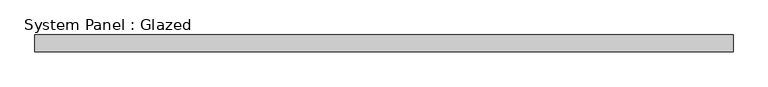
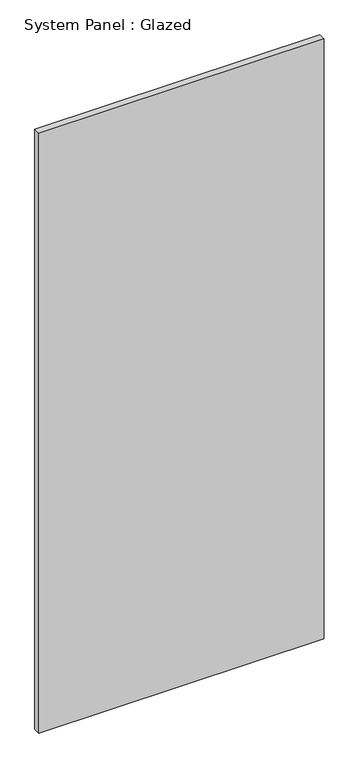
"""IFC4 building model written with IfcOpenShell, lengths in millimetres: plate geometry, System Panel : Glazed."""

from ifc_helpers import new_model, si_unit, origin, origin_with_axes, place, context, project, spatial, polyline, outline, extrude, source, transform, mapped, element, save


def system_panel_glazed_0266aec6(model_context):
    return source(origin(), model_context, "Body", "SweptSolid", [
        extrude(outline(polyline([(527.05, 19.05), (-527.05, 19.05), (-527.05, 44.45), (527.05, 44.45), (527.05, 19.05)])), origin_with_axes(), (0.0, 0.0, 1.0), 2343.15),
    ])


if __name__ == "__main__":
    model = new_model("IFC4")
    model_context = context("Model", 3, world=origin())
    ifc_project = project(units=[si_unit("LENGTHUNIT", "METRE", prefix="MILLI")], contexts=[model_context])
    site = spatial("IfcSite", under=ifc_project)
    building = spatial("IfcBuilding", under=site)
    placement = place(None, origin())
    system_panel_glazed_shape = system_panel_glazed_0266aec6(model_context)
    element("IfcPlate", 1, ObjectType="System Panel : Glazed", at=placement, inside=building, context=model_context, shape_type="MappedRepresentation", body=[
        mapped(system_panel_glazed_shape, transform((0.0, 0.0, 0.0), x_axis=(1.0, 0.0, 0.0), y_axis=(0.0, 1.0, 0.0), z_axis=(0.0, 0.0, 1.0))),
    ])
    save(model, "model.ifc")

# Revit data of these elements
# Type "System Panel : Glazed"
#   Construction Type Id = "GSP4R"
#   Analytic Construction = "1/8 in Pilkington single glazing"
#   Visual Light Transmittance = 0.9
#   Solar Heat Gain Coefficient = 0.86
#   Heat Transfer Coefficient (U) = 1.18115 BTU/(h·ft²·°F)
# Element 1 (IfcPlate, "System Panel : Glazed")
#   Materials on its faces: "Glass"
# Materials
#   "Glass": class "Glass", colour RGB 0 128 192, transparency 0.75, Description = "Soda Lime Glass", Cost = 0
